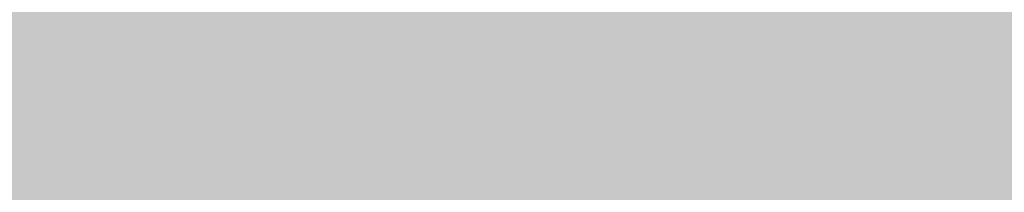
# Model space of a CAD drawing. Units: inches. Extents: x 2091 to 2899, y 967 to 2217.
# Tile 177 of 256: x 2203.151632 to 2203.161218, y 1152.248741 to 1152.250422. Entities that reach past the tile are written whole.
import ezdxf

# ---------------------------------------------------------------- set-up
doc = ezdxf.new("R2010")
doc.units = ezdxf.units.IN
doc.layers.add('A-WALL-PATT', color=141, linetype='Continuous', lineweight=13, true_color=0xadddf7)

msp = doc.modelspace()

# ---------------------------------------------------------------- hatches: boundary and pattern name
at = {"layer": 'A-WALL-PATT'}
h = msp.add_hatch(color=256, dxfattribs=at)
h.dxf.hatch_style = 1
h.paths.add_polyline_path([(2803.1436027, 2050.9190588), (2203.1436027, 2050.9190588), (2203.1436027, 1090.9190588), (2803.1436027, 1090.9190588)])
h.paths.add_polyline_path([(2635.7988501, 1147.5404649), (2674.5240524, 1147.5404649, 0.376086), (2678.5296653, 1152.8802017), (2678.5296653, 1159.5564734, 0.333335), (2674.524319, 1163.561846), (2674.524319, 1163.5618504), (2674.524319, 1192.9343904), (2635.8059707, 1192.9343904), (2597.0876225, 1192.9343904), (2597.0876225, 1163.561846, 0.333335), (2593.0822761, 1159.5564734), (2593.0822761, 1152.8802017, 0.376086), (2597.087889, 1147.5404649)], flags=0)
h.paths.add_polyline_path([(2436.0104329, 1278.2407784, 0.000483), (2435.9526433, 1278.215027, -0.001328), (2435.9356253, 1278.1116934, -0.001711), (2436.1164401, 1278.0407583, 0.002185)], flags=0)
h.paths.add_polyline_path([(2794.1436027, 1143.4190588), (2794.1436027, 1347.4190588), (2543.3701706, 1347.4190588), (2543.3701706, 1351.9190588), (2794.1436027, 1351.9190588), (2794.1436027, 1392.7135549), (2793.9473982, 1392.7135549), (2793.9473982, 1473.5368999), (2794.1436027, 1473.5368999), (2794.1436027, 1531.9190588), (2650.1436027, 1531.9190588), (2650.1436027, 1536.4190588), (2794.1436027, 1536.4190588), (2794.1436027, 1692.4190588), (2609.3756095, 1692.4190588), (2609.3756095, 1644.4190588), (2604.8756095, 1644.4190588), (2604.8756095, 1744.9190588), (2609.3756095, 1744.9190588), (2609.3756095, 1696.9190588), (2794.1436027, 1696.9190588), (2794.1436027, 1780.9190588), (2609.6436027, 1780.9190588), (2493.8756095, 1780.9190588), (2493.8756095, 1785.4190588), (2609.6436027, 1785.4190588), (2794.1436027, 1785.4190588), (2794.1436027, 1847.9388214), (2793.9512217, 1847.9388214), (2793.9512217, 1928.7621663), (2794.1436027, 1928.7621663), (2794.1436027, 1941.4190588), (2614.1436027, 1941.4190588), (2614.1436027, 1821.4190588), (2609.6436027, 1821.4190588), (2609.6436027, 1941.4190588), (2392.1436027, 1941.4190588), (2392.1436027, 1819.9190588), (2387.6436027, 1819.9190588), (2387.6436027, 1941.4190588), (2212.1436027, 1941.4190588), (2212.1436027, 1783.9190588), (2392.1436027, 1783.9190588), (2392.1436027, 1780.9190588), (2212.1436027, 1780.9190588), (2212.1436027, 1629.4190588), (2387.6436027, 1629.4190588), (2387.6436027, 1744.9190588), (2392.1436027, 1744.9190588), (2392.1436027, 1627.9190588), (2317.1436027, 1627.9190588), (2317.1436027, 1551.4190588), (2317.1436027, 1536.4190588), (2459.3835909, 1536.4190588), (2459.3835909, 1602.3964802), (2463.8835909, 1602.3964802), (2463.8835909, 1531.9190588), (2456.6436027, 1531.9190588), (2456.6436027, 1529.9190588), (2452.1436027, 1529.9190588), (2452.1436027, 1531.9190588), (2312.6436027, 1531.9190588), (2312.6436027, 1551.4190588), (2306.1436027, 1551.4190588), (2306.1436027, 1555.9190588), (2308.1436027, 1555.9190588), (2308.1436027, 1551.4190588), (2312.6436027, 1551.4190588), (2312.6436027, 1627.9190588), (2212.1436027, 1627.9190588), (2212.1436027, 1555.9190588), (2270.1436027, 1555.9190588), (2270.1436027, 1551.4190588), (2212.1436027, 1551.4190588), (2212.1436027, 1351.9190588), (2272.1436027, 1351.9190588), (2272.1436027, 1347.4190588), (2212.1436027, 1347.4190588), (2212.1436027, 1275.4190588), (2308.1436027, 1275.4190588), (2308.1436027, 1351.9190588), (2452.1436027, 1351.9190588), (2452.1436027, 1493.9190588), (2456.6436027, 1493.9190588), (2456.6436027, 1347.4190588), (2312.6436027, 1347.4190588), (2312.6436027, 1270.9190588), (2212.1436027, 1270.9190588), (2212.1436027, 1099.9190588), (2281.2375229, 1099.9190588), (2282.8710413, 1110.9138034), (2282.0083413, 1116.9966034), (2278.5577413, 1121.4204034), (2268.2056413, 1128.0562034), (2272.0876413, 1128.0562034), (2273.8129413, 1131.9270034), (2279.4203413, 1134.6919034), (2285.0278413, 1135.2449034), (2287.6158413, 1137.4568034), (2288.0471413, 1138.0098034), (2289.3411413, 1140.7747034), (2291.0665413, 1139.6687034), (2292.3605413, 1135.2449034), (2295.3798413, 1136.9038034), (2296.2425413, 1135.7979034), (2297.1052413, 1133.0330034), (2300.1246413, 1138.0098034), (2303.1439413, 1138.0098034), (2304.4379413, 1135.7979034), (2303.1439413, 1133.5860034), (2306.5946413, 1134.6919034), (2307.8887413, 1133.0330034), (2310.9080413, 1135.2449034), (2313.9274413, 1134.1389034), (2315.6268599, 1132.4271023), (2308.3200413, 1117.5496034), (2290.2038413, 1109.8079034), (2288.9098413, 1103.1721034), (2289.2723086, 1099.9190588), (2434.9182274, 1099.9190588), (2431.5932274, 1124.7880588), (2429.9302274, 1169.5530588), (2430.9271848, 1240.5196942), (2435.6589255, 1238.1861258), (2437.1352274, 1196.5540588), (2438.7982274, 1143.9730588), (2442.6782274, 1111.9980588), (2446.5582274, 1099.9190588), (2794.1436027, 1099.9190588), (2794.1436027, 1138.9190588), (2548.0324471, 1138.9190588), (2548.0324471, 1143.4190588), (2548.0324471, 1148.8190588), (2546.6684571, 1148.0315588), (2528.6856919, 1179.1786218, 0.256256), (2512.0324471, 1148.8190588), (2512.0324471, 1143.4190588), (2512.0324471, 1138.9190588), (2507.5324471, 1138.9190588), (2507.5324471, 1143.4190588), (2507.5324471, 1148.8190588, 0.256256), (2490.8792023, 1179.1786218), (2472.8964371, 1148.0315588), (2471.5324471, 1148.8190588), (2471.5324471, 1143.4190588), (2467.0324471, 1143.4190588), (2467.0324471, 1269.9457858, 0.039061), (2460.9099871, 1273.5800588), (2467.0324471, 1273.5800588), (2467.0324471, 1286.3253638, 0.014511), (2465.2161944, 1286.7619052), (2467.0324471, 1287.0525761), (2467.0324471, 1323.4190588), (2471.5324471, 1323.4190588), (2471.5324471, 1148.8190588), (2489.5324471, 1179.9959734), (2490.8964371, 1179.2084734), (2490.8792023, 1179.1786218, -0.256256), (2507.5324471, 1148.8190588), (2507.5324471, 1143.4190588), (2512.0324471, 1143.4190588), (2512.0324471, 1148.8190588, -0.256256), (2528.6856919, 1179.1786218), (2528.6684571, 1179.2084734), (2530.0324471, 1179.9959734), (2548.0324471, 1148.8190588), (2548.0324471, 1143.4190588)], flags=16)
h.paths.add_polyline_path([(2607.7685461, 1200.9450832), (2607.7685461, 1265.0306251), (2597.0876225, 1281.0520106), (2619.7845852, 1281.0520106), (2627.795278, 1337.1268598), (2635.7988501, 1337.1268598), (2643.8166634, 1337.1268598), (2651.8273562, 1281.0520106), (2674.524319, 1281.0520106), (2663.8433953, 1265.0306251), (2663.8433953, 1200.9450832), (2635.8059707, 1200.9450832)], flags=0)
edge = h.paths.add_edge_path(flags=0)
edge.add_ellipse((13303.8962153, 1272.9987247), major_axis=(-10595.3130399, 0.0000005), ratio=0.842303870086, start_angle=0.62823721906, end_angle=0.64655409989, ccw=False)
edge.add_ellipse((2711.7004495, 1156.8526781), major_axis=(2.2197691, 0), ratio=0.84230387, start_angle=111.5352435, end_angle=180.6282372, ccw=False)
edge.add_ellipse((13303.1562922, 1272.9987246), major_axis=(-10593.0263064, 0), ratio=0.842303869544, start_angle=0.52827147182, end_angle=0.64655409706, ccw=False)
edge.add_line((2710.7645961, 1175.3332951), (2710.1299858, 1175.3332951))
edge.add_ellipse((2710.1299858, 1176.5797752), major_axis=(1.4798461, 0), ratio=0.84230387, start_angle=180, end_angle=270, ccw=False)
edge.add_line((2708.6501397, 1176.5797752), (2708.6501397, 1200.7829144))
edge.add_ellipse((2710.1299858, 1200.7829144), major_axis=(1.4798461, 0), ratio=0.84230387, start_angle=90, end_angle=180, ccw=False)
edge.add_line((2710.1299858, 1202.0293944), (2710.4650752, 1202.0293944))
edge.add_ellipse((13303.1562922, 1272.9987246), major_axis=(-10593.0263064, 0), ratio=0.842303869544, start_angle=-0.09022908859, end_angle=0.38386677879, ccw=False)
edge.add_ellipse((2710.1299858, 1290.9270308), major_axis=(-1.4798461, 0), ratio=0.84230387, start_angle=0, end_angle=90, ccw=False)
edge.add_line((2708.6501397, 1290.9270308), (2708.6501397, 1315.13017))
edge.add_ellipse((2710.1299858, 1315.13017), major_axis=(-1.4798461, 0), ratio=0.84230387, start_angle=-90, end_angle=0, ccw=False)
edge.add_line((2710.1299858, 1316.3766501), (2710.7063141, 1316.3766501))
edge.add_ellipse((3238.4017202, 1296.2895655), major_axis=(528.2339998, 0), ratio=0.84230386954, start_angle=176.349572414, end_angle=177.820049686, ccw=False)
edge.add_ellipse((2775.0630432, 1071.4506962), major_axis=(313.3077613, 0), ratio=0.84230386954, start_angle=102.125965552, end_angle=103.780528989, ccw=False)
edge.add_ellipse((2775.0630432, 1078.3056979), major_axis=(-305.3028915, 0), ratio=0.84230386955, start_angle=-79.790461003, end_angle=-77.555372706, ccw=False)
edge.add_ellipse((2695.1417666, 1541.9753825), major_axis=(-250.9602162, 0), ratio=0.84230386954, start_angle=99.256566007, end_angle=102.554932644)
edge.add_line((2741.4103262, 1334.2142554), (2747.1325454, 1337.3784768))
edge.add_ellipse((2747.5386163, 1336.8574776), major_axis=(-0.739923, 0), ratio=0.84230387, start_angle=270, end_angle=307.9331305, ccw=False)
edge.add_ellipse((2747.5386163, 1336.8574776), major_axis=(-0.739923, 0), ratio=0.84230387, start_angle=232.0668695, end_angle=270, ccw=False)
edge.add_line((2747.9446872, 1337.3784768), (2753.6669064, 1334.2142554))
edge.add_ellipse((2799.935466, 1541.9753825), major_axis=(250.9602162, 0), ratio=0.84230386954, start_angle=257.445067356, end_angle=260.743433993)
edge.add_ellipse((2720.0141894, 1078.3056979), major_axis=(305.3028915, 0), ratio=0.84230386954, start_angle=77.555372707, end_angle=79.790461003, ccw=False)
edge.add_ellipse((2720.0141894, 1071.4506962), major_axis=(-313.3077613, 0), ratio=0.84230386954, start_angle=256.219471011, end_angle=257.874034448, ccw=False)
edge.add_ellipse((2256.6755124, 1296.2895655), major_axis=(-528.2339998, 0), ratio=0.84230386954, start_angle=182.179950314, end_angle=183.650427586, ccw=False)
edge.add_line((2784.3709184, 1316.3766501), (2784.9472468, 1316.3766501))
edge.add_ellipse((2784.9472468, 1315.13017), major_axis=(1.4798461, 0), ratio=0.84230387, start_angle=0, end_angle=90, ccw=False)
edge.add_line((2786.4270928, 1315.13017), (2786.4270928, 1290.9270308))
edge.add_ellipse((2784.9472468, 1290.9270308), major_axis=(1.4798461, 0), ratio=0.84230387, start_angle=270, end_angle=360, ccw=False)
edge.add_ellipse((-7808.0790596, 1272.9987246), major_axis=(10593.0263063, 0), ratio=0.842303869544, start_angle=-0.38386677879, end_angle=0.09022908859, ccw=False)
edge.add_line((2784.6121574, 1202.0293944), (2784.9472468, 1202.0293944))
edge.add_ellipse((2784.9472468, 1200.7829144), major_axis=(1.4798461, 0), ratio=0.84230387, start_angle=0, end_angle=90, ccw=False)
edge.add_line((2786.4270928, 1200.7829144), (2786.4270928, 1176.5797752))
edge.add_ellipse((2784.9472468, 1176.5797752), major_axis=(-1.4798461, 0), ratio=0.84230387, start_angle=90, end_angle=180, ccw=False)
edge.add_line((2784.9472468, 1175.3332951), (2784.3126365, 1175.3332951))
edge.add_ellipse((-7808.0790596, 1272.9987246), major_axis=(10593.0263063, 0), ratio=0.842303869544, start_angle=-0.61864319632, end_angle=-0.52827147182, ccw=False)
edge.add_ellipse((2783.3767831, 1156.8526781), major_axis=(-2.2197691, 0), ratio=0.84230387, start_angle=179.3717628, end_angle=248.4647566, ccw=False)
edge.add_ellipse((-7808.8189826, 1272.9987246), major_axis=(-10595.3130398, 0.0000036), ratio=0.842303865762, start_angle=179.3534459226, end_angle=179.37176280343, ccw=False)
edge.add_ellipse((2780.2973026, 1153.500793), major_axis=(-5.2464256, 0), ratio=0.84230387, start_angle=90, end_angle=179.3534459, ccw=False)
edge.add_line((2780.2973026, 1149.0817084), (2714.77993, 1149.0817084))
edge.add_ellipse((2714.77993, 1153.500793), major_axis=(5.2464256, 0), ratio=0.84230387, start_angle=180.6465541, end_angle=270, ccw=False)
edge = h.paths.add_edge_path(flags=0)
edge.add_line((2718.1873674, 1151.0078329), (2718.1873674, 1170.4723638))
edge.add_ellipse((2721.1470595, 1170.4723638), major_axis=(-2.9596921, 0), ratio=0.84230387, start_angle=-90, end_angle=0, ccw=False)
edge.add_line((2721.1470595, 1172.965324), (2773.9301731, 1172.965324))
edge.add_ellipse((2773.9301731, 1170.4723638), major_axis=(-2.9596921, 0), ratio=0.84230387, start_angle=180, end_angle=270, ccw=False)
edge.add_line((2776.8898652, 1170.4723638), (2776.8898652, 1151.0078329))
edge.add_line((2776.8898652, 1151.0078329), (2718.1873674, 1151.0078329))
edge = h.paths.add_edge_path(flags=0)
edge.add_line((2718.1873674, 1180.2341502), (2718.1873674, 1199.0578342))
edge.add_ellipse((2747.5386163, 1320.3986402), major_axis=(147.0179239, 0), ratio=0.84230386954, start_angle=256.40186531, end_angle=283.59813469)
edge.add_line((2776.8898652, 1199.0578342), (2776.8898652, 1180.2341502))
edge.add_ellipse((2747.5386163, 1301.5749562), major_axis=(147.0179239, 0), ratio=0.84230386954, start_angle=256.40186531, end_angle=283.59813469, ccw=False)
edge = h.paths.add_edge_path(flags=0)
edge.add_ellipse((13303.1562922, 1272.9987246), major_axis=(-10591.5464603, 0), ratio=0.842303869555, start_angle=0.05559431352, end_angle=0.37776419393, ccw=False)
edge.add_line((2711.6168595, 1262.7217103), (2715.6674076, 1249.4953957))
edge.add_ellipse((6413.8919626, 1241.691919), major_axis=(-3698.2361592, 0), ratio=0.842303869547, start_angle=-0.120897369, end_angle=0.3640763489)
edge.add_line((2715.7610383, 1218.1924547), (2711.9343065, 1203.167361))
edge = h.paths.add_edge_path(flags=0)
edge.add_line((2718.1873674, 1251.074566), (2716.0024854, 1267.4504351))
edge.add_ellipse((2742.1511746, 1202.1895399), major_axis=(81.7725845, 0), ratio=0.8423038695, start_angle=94.277420963, end_angle=111.834953797, ccw=False)
edge.add_line((2737.0097482, 1270.9306255), (2758.0674844, 1270.9306255))
edge.add_ellipse((2752.926058, 1202.1895399), major_axis=(81.7725845, 0), ratio=0.8423038695, start_angle=68.165046203, end_angle=85.722579037, ccw=False)
edge.add_line((2779.0747472, 1267.4504351), (2776.8898652, 1251.074566))
edge.add_ellipse((2750.3380588, 1187.8853558), major_axis=(79.5796641, 0), ratio=0.8423038695, start_angle=67.208085122, end_angle=85.129930403)
edge.add_line((2756.0346562, 1254.7436557), (2739.0425764, 1254.7436557))
edge.add_ellipse((2744.7391738, 1187.8853558), major_axis=(79.5796641, 0), ratio=0.8423038695, start_angle=94.870069597, end_angle=112.791914878)
edge = h.paths.add_edge_path(flags=0)
edge.add_line((2783.1429261, 1203.167361), (2779.3161943, 1218.1924547))
edge.add_ellipse((-918.81473, 1241.691919), major_axis=(3698.2361592, 0), ratio=0.842303869546, start_angle=-0.3640763489, end_angle=0.120897369)
edge.add_line((2779.409825, 1249.4953957), (2783.4603731, 1262.7217103))
edge.add_ellipse((-7808.0790596, 1272.9987246), major_axis=(-10591.5464603, 0), ratio=0.84230386954, start_angle=179.6222358061, end_angle=179.94440568651, ccw=False)
edge = h.paths.add_edge_path(flags=0)
edge.add_ellipse((2734.2008921, 1286.6904402), major_axis=(-0.3566086, 6.3400775), ratio=0.603833576, start_angle=89.00201428, end_angle=253.65740805, ccw=False)
edge.add_line((2730.3690013, 1286.5418057), (2730.3690013, 1301.3519803))
edge.add_line((2730.3690013, 1301.3519803), (2735.9133107, 1305.2148028))
edge.add_ellipse((2736.3849168, 1304.7345612), major_axis=(0.739923, 0), ratio=0.84230387, start_angle=90, end_angle=134.4802109, ccw=False)
edge.add_line((2736.3849168, 1305.3578013), (2738.0327829, 1305.3578013))
edge.add_line((2738.0327829, 1305.3578013), (2738.0327829, 1307.7079274))
edge.add_ellipse((2794.201642, 1307.7079274), major_axis=(56.168859, 0), ratio=0.8423038695, start_angle=150.5614304, end_angle=180, ccw=False)
edge.add_ellipse((2700.8755906, 1307.7079274), major_axis=(-56.168859, 0), ratio=0.8423038695, start_angle=180, end_angle=209.4385696, ccw=False)
edge.add_line((2757.0444497, 1307.7079274), (2757.0444497, 1305.3578013))
edge.add_line((2757.0444497, 1305.3578013), (2758.6923157, 1305.3578013))
edge.add_ellipse((2758.6923157, 1304.7345612), major_axis=(-0.739923, 0), ratio=0.84230387, start_angle=225.5197891, end_angle=270, ccw=False)
edge.add_line((2759.1639219, 1305.2148028), (2764.7082312, 1301.3519803))
edge.add_line((2764.7082312, 1301.3519803), (2764.7082312, 1286.5418057))
edge.add_ellipse((2760.8763405, 1286.6904402), major_axis=(0.3566086, 6.3400775), ratio=0.603833576, start_angle=106.34259195, end_angle=270.99798572, ccw=False)
edge.add_line((2757.0444497, 1285.7970896), (2757.0444497, 1307.7079274))
edge.add_ellipse((2700.8755906, 1307.7079274), major_axis=(-56.168859, 0), ratio=0.8423038695, start_angle=180, end_angle=209.4385696)
edge.add_ellipse((2794.201642, 1307.7079274), major_axis=(56.168859, 0), ratio=0.8423038695, start_angle=150.5614304, end_angle=180)
edge.add_line((2738.0327829, 1307.7079274), (2738.0327829, 1285.7970896))
h.paths.add_polyline_path([(2417.8122727, 1104.449704), (2413.4922727, 1102.529704), (2410.6122727, 1103.969704), (2409.1722727, 1106.369704), (2407.2522727, 1107.329704), (2406.2922727, 1109.729704), (2405.3322727, 1114.049704), (2405.3322727, 1117.889704), (2406.2922727, 1120.129704), (2407.2522727, 1119.809704), (2408.8483218, 1118.3276585), (2410.1739451, 1119.4241703), (2410.2112727, 1120.405704), (2411.0407305, 1121.4190541), (2410.6992727, 1119.858704), (2410.1739451, 1119.4241703), (2410.0884515, 1117.1761095), (2411.1328361, 1116.2063237), (2413.9722727, 1119.329704), (2416.8522727, 1120.769704), (2416.8697209, 1120.7987842), (2417.0350713, 1119.4051162), (2417.8962134, 1118.1433844), (2418.2922727, 1118.369704), (2419.5444467, 1120.0392692), (2419.3609153, 1118.387487), (2419.0321078, 1119.3561507), (2418.3989394, 1118.5119262), (2419.2522727, 1114.529704), (2418.7940909, 1107.1987949)], flags=0)
h.paths.add_polyline_path([(2508.8701706, 1347.4190588), (2508.3701706, 1347.4190588), (2508.3701706, 1351.9190588), (2508.8701706, 1351.9190588)], flags=0)
h.paths.add_polyline_path([(2473.3701706, 1347.4190588), (2472.3701706, 1347.4190588), (2467.8701706, 1347.4190588), (2467.8701706, 1455.4190588), (2472.3701706, 1455.4190588), (2472.3701706, 1352.4190588), (2473.3701706, 1352.4190588)], flags=0)
h.paths.add_polyline_path([(2352.106244, 1217.4461971), (2349.226244, 1218.8861971), (2347.786244, 1221.2861971), (2345.866244, 1222.2461971), (2344.906244, 1224.6461971), (2343.946244, 1228.9661971), (2343.946244, 1232.8061971), (2344.906244, 1235.0461971), (2345.866244, 1234.7261971), (2347.4622931, 1233.2441515), (2348.7879164, 1234.3406634), (2348.825244, 1235.3221971), (2349.6547018, 1236.3355471), (2349.313244, 1234.7751971), (2348.7879164, 1234.3406634), (2348.7024228, 1232.0926025), (2349.7468074, 1231.1228168), (2352.586244, 1234.2461971), (2355.466244, 1235.6861971), (2355.4836921, 1235.7152773), (2355.6490426, 1234.3216093), (2356.5101846, 1233.0598774), (2356.906244, 1233.2861971), (2358.1584179, 1234.9557623), (2357.9748866, 1233.3039801), (2357.6460791, 1234.2726438), (2357.0129107, 1233.4284193), (2357.866244, 1229.4461971), (2357.4080622, 1222.115288), (2356.426244, 1219.3661971)], flags=0)
h.paths.add_polyline_path([(2348.2967999, 1112.2244204), (2347.0137999, 1112.3104204), (2345.5297999, 1114.1274204), (2345.7317999, 1115.8584204), (2346.8117999, 1116.9824204), (2346.8117999, 1114.6464204), (2345.8667999, 1114.2144204), (2346.8797999, 1114.3004204)], flags=0)
h.paths.add_polyline_path([(2347.0137999, 1110.9264204), (2346.2717999, 1110.4934204), (2346.6097999, 1111.1864204)], flags=0)
h.paths.add_polyline_path([(2345.8667999, 1118.1944204), (2345.5297999, 1117.3294204), (2343.7077999, 1118.0214204), (2344.3827999, 1118.6264204)], flags=0)
h.paths.add_polyline_path([(2346.6767999, 1109.2824204), (2346.0697999, 1108.0714204), (2345.8667999, 1110.0614204)], flags=0)
h.paths.add_polyline_path([(2345.0567999, 1119.7514204), (2343.6397999, 1119.7514204), (2343.9777999, 1121.1354204)], flags=0)
h.paths.add_polyline_path([(2345.2597999, 1116.5504204), (2345.1247999, 1115.8584204), (2344.9217999, 1115.6854204), (2344.7197999, 1116.3774204)], flags=0)
h.paths.add_polyline_path([(2345.6647999, 1112.3104204), (2345.4617999, 1111.5324204), (2344.0447999, 1111.9644204), (2344.6517999, 1112.5704204)], flags=0)
h.paths.add_polyline_path([(2345.1917999, 1113.3494204), (2344.4497999, 1113.8684204), (2344.7197999, 1114.3874204)], flags=0)
h.paths.add_polyline_path([(2344.6517999, 1116.8094204), (2344.1797999, 1115.6854204), (2344.6517999, 1115.3394204), (2343.9097999, 1114.9064204), (2343.0327999, 1115.9444204), (2343.6397999, 1116.4634204)], flags=0)
h.paths.add_polyline_path([(2345.8667999, 1106.6864204), (2344.9897999, 1105.5624204), (2344.5167999, 1106.6004204)], flags=0)
h.paths.add_polyline_path([(2344.8547999, 1110.0614204), (2344.5167999, 1109.2824204), (2344.1127999, 1109.7154204)], flags=0)
h.paths.add_polyline_path([(2344.0447999, 1113.5224204), (2343.4377999, 1113.0894204), (2342.7627999, 1113.9544204)], flags=0)
h.paths.add_polyline_path([(2344.3147999, 1111.0124204), (2342.9647999, 1110.3204204), (2342.9647999, 1111.0994204)], flags=0)
h.paths.add_polyline_path([(2345.1247999, 1104.6974204), (2344.5847999, 1103.7454204), (2344.4497999, 1104.2644204)], flags=0)
h.paths.add_polyline_path([(2342.8297999, 1121.2224204), (2341.7497999, 1120.5304204), (2340.5357999, 1121.0494204), (2340.1307999, 1121.8284204), (2340.6707999, 1122.9524204), (2341.1427999, 1121.8284204), (2341.6147999, 1122.0014204)], flags=0)
h.paths.add_polyline_path([(2342.9647999, 1119.7514204), (2343.0327999, 1118.4534204), (2342.0877999, 1118.0214204), (2342.0197999, 1119.4914204)], flags=0)
h.paths.add_polyline_path([(2342.6947999, 1116.8964204), (2341.9527999, 1116.6364204), (2342.0197999, 1117.3294204)], flags=0)
h.paths.add_polyline_path([(2343.0327999, 1112.2244204), (2342.0197999, 1111.7914204), (2341.5477999, 1112.2244204), (2342.3577999, 1113.3494204)], flags=0)
h.paths.add_polyline_path([(2343.7747999, 1104.4374204), (2342.6277999, 1102.8804204), (2342.6947999, 1104.6104204), (2343.4377999, 1105.1294204)], flags=0)
h.paths.add_polyline_path([(2342.0197999, 1115.0794204), (2340.8057999, 1115.5124204), (2340.9407999, 1116.3774204)], flags=0)
h.paths.add_polyline_path([(2341.4807999, 1120.0974204), (2341.4807999, 1119.4054204), (2341.0757999, 1119.5784204), (2341.1427999, 1120.0974204)], flags=0)
h.paths.add_polyline_path([(2341.8177999, 1114.4734204), (2340.9407999, 1113.0894204), (2340.8057999, 1114.5604204)], flags=0)
h.paths.add_polyline_path([(2341.1427999, 1118.5404204), (2340.9407999, 1116.9824204), (2339.0507999, 1117.6754204), (2339.0507999, 1118.6264204)], flags=0)
h.paths.add_polyline_path([(2342.6947999, 1101.6684204), (2341.9527999, 1101.8414204), (2342.5597999, 1102.3614204)], flags=0)
h.paths.add_polyline_path([(2340.3327999, 1119.6654204), (2338.4437999, 1119.5784204), (2337.9037999, 1120.3574204), (2339.6577999, 1120.6164204)], flags=0)
h.paths.add_polyline_path([(2340.3327999, 1115.3394204), (2340.0627999, 1113.6954204), (2339.3877999, 1115.3394204)], flags=0)
h.paths.add_polyline_path([(2341.8177999, 1103.8314204), (2341.5477999, 1102.8804204), (2341.1427999, 1103.6584204)], flags=0)
h.paths.add_polyline_path([(2339.0507999, 1122.8664204), (2337.2957999, 1121.8284204), (2337.0937999, 1123.1254204), (2337.7687999, 1123.8184204)], flags=0)
h.paths.add_polyline_path([(2339.1177999, 1121.7414204), (2338.8477999, 1121.2224204), (2338.1737999, 1121.0494204), (2338.3757999, 1121.5684204)], flags=0)
h.paths.add_polyline_path([(2339.1857999, 1119.3194204), (2338.6457999, 1118.7134204), (2338.2407999, 1118.1074204), (2338.2407999, 1118.8864204)], flags=0)
h.paths.add_polyline_path([(2341.1427999, 1101.9284204), (2340.6027999, 1101.2364204), (2340.0627999, 1101.8414204), (2340.6027999, 1102.3614204)], flags=0)
h.paths.add_polyline_path([(2337.6337999, 1117.7614204), (2336.6207999, 1118.2804204), (2337.2957999, 1118.9724204)], flags=0)
h.paths.add_polyline_path([(2336.8237999, 1119.5784204), (2334.7987999, 1118.9724204), (2335.2037999, 1120.3574204), (2336.5537999, 1120.8764204)], flags=0)
h.paths.add_polyline_path([(2339.1177999, 1100.4574204), (2337.3637999, 1100.5434204), (2336.7557999, 1101.2364204)], flags=0)
h.paths.add_polyline_path([(2336.3507999, 1122.4334204), (2336.0137999, 1121.9144204), (2334.9337999, 1122.4334204), (2334.5287999, 1123.4714204), (2335.7437999, 1122.7794204)], flags=0)
h.paths.add_polyline_path([(2334.7317999, 1120.8764204), (2334.2587999, 1120.3574204), (2334.0567999, 1120.7894204), (2334.5967999, 1121.3084204)], flags=0)
h.paths.add_polyline_path([(2334.4617999, 1122.1744204), (2332.5717999, 1121.3084204), (2331.3567999, 1122.1744204), (2332.0997999, 1122.8664204)], flags=0)
h.paths.add_polyline_path([(2334.2587999, 1118.5404204), (2333.3817999, 1118.4534204), (2333.6517999, 1119.3194204)], flags=0)
h.paths.add_polyline_path([(2335.5417999, 1102.2744204), (2334.1917999, 1102.6204204), (2335.2717999, 1103.3124204)], flags=0)
h.paths.add_polyline_path([(2332.7067999, 1119.6654204), (2331.6947999, 1120.4434204), (2332.5047999, 1120.7894204)], flags=0)
h.paths.add_polyline_path([(2334.7317999, 1101.1494204), (2333.5167999, 1101.5824204), (2333.9887999, 1101.7554204)], flags=0)
h.paths.add_polyline_path([(2332.6397999, 1116.6364204), (2331.0867999, 1116.2904204), (2331.9647999, 1118.1944204)], flags=0)
h.paths.add_polyline_path([(2330.7497999, 1121.5684204), (2330.2767999, 1120.2704204), (2328.5227999, 1119.3194204), (2328.9947999, 1121.0494204)], flags=0)
h.paths.add_polyline_path([(2330.7497999, 1118.6264204), (2330.0077999, 1117.5024204), (2329.8727999, 1118.0214204)], flags=0)
h.paths.add_polyline_path([(2332.0997999, 1102.3614204), (2330.5467999, 1102.0144204), (2331.6947999, 1102.9664204)], flags=0)
h.paths.add_polyline_path([(2329.5347999, 1113.6084204), (2329.0627999, 1112.3104204), (2328.5897999, 1113.3494204)], flags=0)
h.paths.add_polyline_path([(2328.3877999, 1117.8484204), (2327.5097999, 1116.5504204), (2327.1727999, 1117.7614204)], flags=0)
h.paths.add_polyline_path([(2329.7377999, 1106.5134204), (2329.5347999, 1105.3024204), (2328.2527999, 1106.0814204)], flags=0)
h.paths.add_polyline_path([(2328.6577999, 1114.3874204), (2328.0497999, 1114.1274204), (2328.3197999, 1114.9064204)], flags=0)
h.paths.add_polyline_path([(2328.3197999, 1112.2244204), (2327.1057999, 1112.1374204), (2326.7007999, 1112.6564204)], flags=0)
h.paths.add_polyline_path([(2326.9027999, 1115.2524204), (2326.7007999, 1114.1274204), (2325.2157999, 1113.6084204), (2326.0927999, 1115.3394204)], flags=0)
h.paths.add_polyline_path([(2326.6327999, 1108.3304204), (2326.0927999, 1107.3794204), (2325.8907999, 1108.5034204), (2326.4977999, 1109.1094204)], flags=0)
h.paths.add_polyline_path([(2615.1436027, 1531.9190588), (2609.6436027, 1531.9190588), (2609.6436027, 1620.4190588), (2614.1436027, 1620.4190588), (2614.1436027, 1536.4190588), (2615.1436027, 1536.4190588)], flags=0)
h.paths.add_polyline_path([(2545.1436027, 1563.4190588), (2464.1436027, 1563.4190588), (2464.1436027, 1632.4190588), (2509.1436027, 1632.4190588), (2509.1436027, 1627.9190588), (2509.1436027, 1603.9190588), (2468.6436027, 1603.9190588), (2468.6436027, 1567.9190588), (2540.6436027, 1567.9190588), (2540.6436027, 1591.9190588), (2545.1436027, 1591.9190588)], flags=0)
h.paths.add_polyline_path([(2388.9690483, 1549.985735), (2357.4341811, 1549.985735), (2357.4341811, 1623.3607783), (2399.3627772, 1623.3607783), (2435.6894654, 1623.3607783), (2435.5925469, 1602.5592734), (2435.5925469, 1602.3964802), (2388.9690483, 1602.3964802)], flags=0)
h.paths.add_polyline_path([(2388.8806282, 1555.8091511), (2374.9044295, 1555.8091511), (2374.9044295, 1600.5715641), (2374.9044295, 1615.4576454), (2406.3508766, 1615.4576454), (2406.3508766, 1618.9394309), (2412.1742927, 1615.4576454), (2406.3508766, 1611.9758599), (2406.3508766, 1615.4576454), (2388.8806282, 1615.4576454)], flags=0)
h.paths.add_polyline_path([(2568.8756095, 1644.4190588), (2453.3756095, 1644.4190588), (2453.3756095, 1785.4190588), (2457.8756095, 1785.4190588), (2457.8756095, 1648.9190588), (2568.8756095, 1648.9190588)], flags=0)
h.paths.add_polyline_path([(2212.1436027, 1945.9190588), (2212.1436027, 2041.9190588), (2794.1436027, 2041.9190588), (2794.1436027, 1945.9190588)], flags=16)
h.paths.add_polyline_path([(2271.0827276, 1964.3172377), (2776.852968, 1964.3172377), (2776.852968, 2037.1696226), (2271.0827276, 2037.1696226)], flags=8)
h.paths.add_polyline_path([(2380.6492852, 1536.8241435), (2461.0408087, 1536.8241435), (2461.0408087, 1554.6525871), (2380.6492852, 1554.6525871)], flags=8)
h.paths.add_polyline_path([(2240.7557092, 1609.7254508), (2309.1858294, 1609.7254508), (2309.1858294, 1617.6982037), (2240.7557092, 1617.6982037)], flags=8)
h.paths.add_polyline_path([(2212.6772554, 1313.5041021), (2282.5915203, 1313.5041021), (2282.5915203, 1322.7452389), (2212.6772554, 1322.7452389)], flags=8)
h.paths.add_polyline_path([(2457.111976, 1114.778574), (2558.4815807, 1114.778574), (2558.4815807, 1142.2196823), (2457.111976, 1142.2196823)], flags=8)
h.paths.add_polyline_path([(2473.4423372, 1273.0100672), (2604.6412257, 1273.0100672), (2604.6412257, 1318.3469349), (2473.4423372, 1318.3469349)], flags=8)
h.paths.add_polyline_path([(2638.8763024, 1626.9774316), (2684.2503675, 1627.9767377), (2684.0384825, 1637.5974944), (2638.6644174, 1636.5981884)], flags=8)
h.paths.add_polyline_path([(2537.5905538, 1453.7934466), (2628.3895472, 1453.7934466), (2628.3895472, 1475.3448114), (2537.5905538, 1475.3448114)], flags=8)
h.paths.add_polyline_path([(2504.1376376, 1714.6323972), (2554.6471875, 1714.6323972), (2554.6471875, 1730.2377115), (2504.1376376, 1730.2377115)], flags=8)
h.paths.add_polyline_path([(2487.5011806, 1575.6518716), (2535.0971214, 1575.6518716), (2535.0971214, 1598.3776456), (2487.5011806, 1598.3776456)], flags=8)
h.paths.add_polyline_path([(2709.0994004, 1735.7102784), (2740.0166009, 1735.7102784), (2740.0166009, 1749.9376406), (2709.0994004, 1749.9376406)], flags=8)
h.paths.add_polyline_path([(2442.4384239, 1792.1716575), (2564.7288353, 1792.1716575), (2564.7288353, 1842.0001626), (2442.4384239, 1842.0001626)], flags=8)
h.paths.add_polyline_path([(2655.8158012, 1809.6440763), (2789.5201425, 1806.6937963), (2790.0849768, 1832.2916379), (2656.3806355, 1835.2419179)], flags=8)
h.paths.add_polyline_path([(2234.8426972, 1797.7201432), (2368.5928512, 1794.7688523), (2369.1607182, 1820.504132), (2235.4105642, 1823.4554229)], flags=8)
h.paths.add_polyline_path([(2245.1384659, 1644.0063348), (2398.4277329, 1640.6238997), (2398.9948417, 1666.3248199), (2245.7055747, 1669.7072549)], flags=8)
h.paths.add_polyline_path([(2306.1428474, 1431.1685186), (2413.7683138, 1428.7936873), (2414.3331481, 1454.3915289), (2306.7076817, 1456.7663602)], flags=8)
h.paths.add_polyline_path([(2306.834582, 1458.2331447), (2393.3804836, 1456.3234487), (2393.9328082, 1481.3543583), (2307.3869066, 1483.2640542)], flags=8)

doc.saveas('drawing.dxf')
